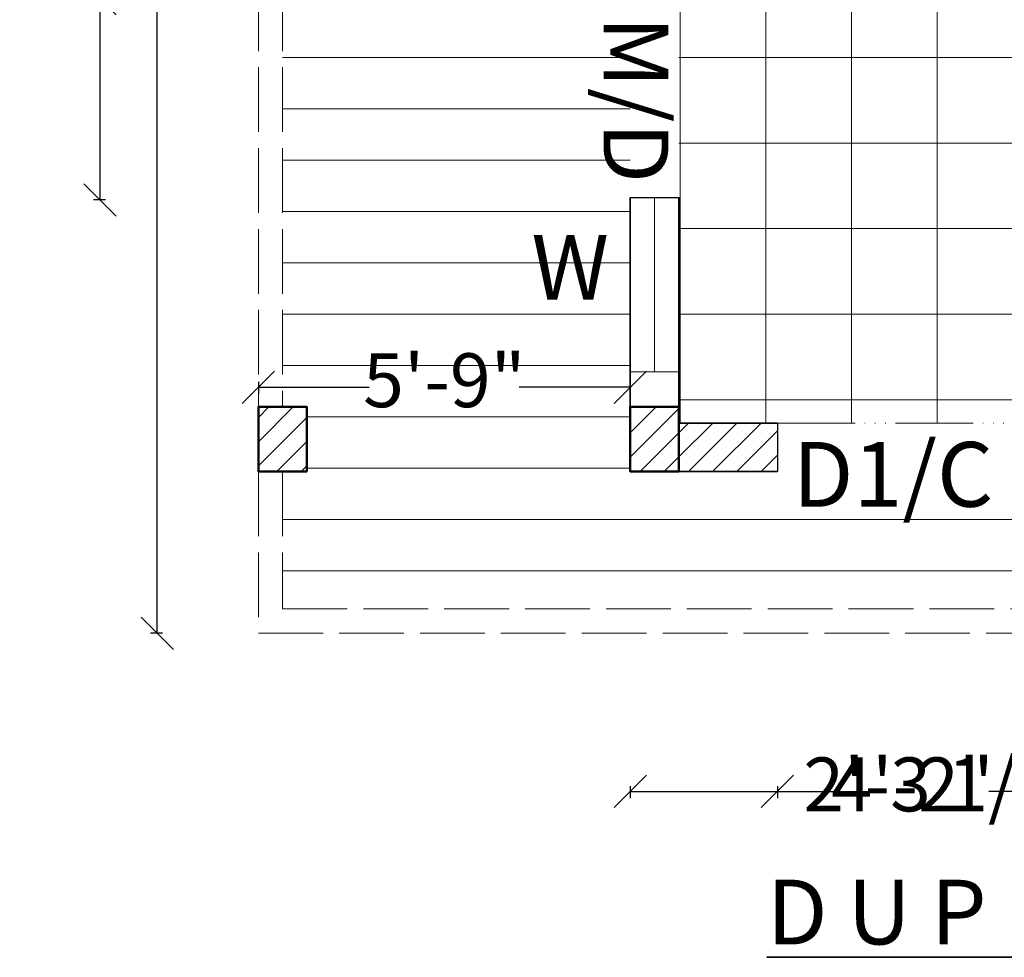
# Model space of a CAD drawing. Units: inches. Extents: x 2036 to 2670, y 319 to 920.
# Tile 1 of 15: x 2036 to 2219, y 405 to 579. Entities that reach past the tile are written whole.
import ezdxf

# ---------------------------------------------------------------- set-up
doc = ezdxf.new("R2010")
doc.units = ezdxf.units.IN
doc.linetypes.add('ACAD_ISO02W100', pattern=[15, 12, -3])
doc.linetypes.add('ACAD_ISO06W100', pattern=[36, 24, -3, 0, -3, 0, -3, 0, -3])
for name, color, linetype, lineweight in [('A-ANNO-DIMS', 2, 'Continuous', 18), ('A-ANNO-TEXT', 7, 'Continuous', 18), ('A-ANNO-TITL', 7, 'Continuous', 35), ('A-COLS', 7, 'Continuous', 50), ('A-DOOR', 3, 'Continuous', 25), ('A-DOOR-OVHD', 3, 'ACAD_ISO06W100', 18), ('A-FLOR-OVHD', 1, 'ACAD_ISO02W100', 13), ('A-FLOR-PATT', 8, 'Continuous', 9), ('A-GLAZ', 4, 'Continuous', 18), ('A-WALL', 7, 'Continuous', 35)]:
    doc.layers.add(name, color=color, linetype=linetype, lineweight=lineweight)
doc.layers.add('A-COLS-PATT', color=240, linetype='Continuous', lineweight=13, true_color=0xed1f24)
doc.layers.add('A-WALL-PATT', color=52, linetype='Continuous', lineweight=13, true_color=0xc8c92d)
doc.styles.get("Standard").update_dxf_attribs({"font": 'arial.ttf'})
doc.dimstyles.new('ISO-25', dxfattribs={"dimtxt": 10, "dimasz": 6, "dimexe": 1.25, "dimexo": 0.625, "dimtad": 0, "dimdec": 1, "dimlunit": 3, "dimtxsty": 'Standard', "dimblk": 'OBLIQUE', "dimcen": 2.5, "dimclrd": 94, "dimclre": 94, "dimclrt": 1, "dimadec": 0, "dimazin": 0, "dimtfac": 1, "dimtdec": 1, "dimtmove": 0, "dimatfit": 3, "dimfxl": 1, "dimfxlon": 1, "dimarcsym": 0})

# ---------------------------------------------------------------- blocks, each defined once
blk = doc.blocks.new('_Oblique')
at = {"color": 0, "linetype": 'ByBlock', "lineweight": -2}
blk.add_line((-0.5, -0.5), (0.5, 0.5), dxfattribs=at)
blk = doc.blocks.new('*D13')
at = {"layer": 'A-ANNO-DIMS', "color": 0, "lineweight": -2, "transparency": 16777216}
for p, q in [((2062.98, 875.68), (2060.73, 875.68)), ((2061.98, 875.68), (2061.98, 687.98)), ((2061.98, 464.68), (2061.98, 652.39)), ((2062.98, 464.68), (2060.73, 464.68))]:
    blk.add_line(p, q, dxfattribs=at)
at = {"layer": 'Defpoints', "color": 0, "transparency": 16777216}
for p in [(2080.74, 875.68), (2061.98, 464.68), (2080.74, 464.68)]:
    blk.add_point(p, dxfattribs=at)
at = {"layer": 'A-ANNO-DIMS', "color": 0, "lineweight": -2, "transparency": 16777216, "xscale": 6, "yscale": 6, "zscale": 6}
for p, rotation in [((2061.98, 875.68), 90), ((2061.98, 464.68), 270)]:
    blk.add_blockref('_Oblique', p, dxfattribs=dict(at, rotation=rotation))
at = {"layer": 'A-ANNO-DIMS', "color": 0, "transparency": 16777216, "insert": (2061.98, 670.18), "char_height": 10, "attachment_point": 5, "rotation": 90}
blk.add_mtext('34\'-3"', dxfattribs=at)
blk = doc.blocks.new('*D15')
at = {"layer": 'A-ANNO-DIMS', "color": 0, "lineweight": -2, "transparency": 16777216}
for p, q in [((2080.74, 511.32), (2080.74, 509.07)), ((2080.74, 510.32), (2101.32, 510.32)), ((2149.74, 510.32), (2129.15, 510.32)), ((2149.74, 511.32), (2149.74, 509.07))]:
    blk.add_line(p, q, dxfattribs=at)
at = {"layer": 'Defpoints', "color": 0, "transparency": 16777216}
for p in [(2080.74, 514.8), (2149.74, 514.8), (2149.74, 510.32)]:
    blk.add_point(p, dxfattribs=at)
at = {"layer": 'A-ANNO-DIMS', "color": 0, "lineweight": -2, "transparency": 16777216, "xscale": 6, "yscale": 6, "zscale": 6, "rotation": 180}
blk.add_blockref('_Oblique', (2080.74, 510.32), dxfattribs=at)
at = {"layer": 'A-ANNO-DIMS', "color": 0, "lineweight": -2, "transparency": 16777216, "xscale": 6, "yscale": 6, "zscale": 6}
blk.add_blockref('_Oblique', (2149.74, 510.32), dxfattribs=at)
at = {"layer": 'A-ANNO-DIMS', "color": 0, "transparency": 16777216, "insert": (2115.24, 510.32), "char_height": 10, "attachment_point": 5}
blk.add_mtext('5\'-9"', dxfattribs=at)
blk = doc.blocks.new('COL-9x12')
blk.add_lwpolyline([(9, 0), (0, 0), (0, 12), (9, 12)], close=True)
blk = doc.blocks.new('*D41')
at = {"layer": 'A-ANNO-DIMS', "color": 94, "lineweight": -2, "transparency": 16777216}
for p, q in [((2149.74, 436.33), (2149.74, 434.08)), ((2149.74, 435.33), (2177.02, 435.33)), ((2177.02, 436.33), (2177.02, 434.08)), ((2177.02, 435.33), (2183.02, 435.33))]:
    blk.add_line(p, q, dxfattribs=at)
at = {"layer": 'Defpoints', "color": 0, "transparency": 16777216}
for p in [(2149.74, 494.68), (2177.02, 494.68), (2177.02, 435.33)]:
    blk.add_point(p, dxfattribs=at)
at = {"layer": 'A-ANNO-DIMS', "color": 94, "lineweight": -2, "transparency": 16777216, "xscale": 6, "yscale": 6, "zscale": 6, "rotation": 180}
blk.add_blockref('_Oblique', (2149.74, 435.33), dxfattribs=at)
at = {"layer": 'A-ANNO-DIMS', "color": 94, "lineweight": -2, "transparency": 16777216, "xscale": 6, "yscale": 6, "zscale": 6}
blk.add_blockref('_Oblique', (2177.02, 435.33), dxfattribs=at)
at = {"layer": 'A-ANNO-DIMS', "color": 1, "transparency": 16777216, "insert": (2208.67, 435.33), "char_height": 10, "attachment_point": 5}
blk.add_mtext('2\'-3 1/2"', dxfattribs=at)
blk = doc.blocks.new('*D42')
at = {"layer": 'A-ANNO-DIMS', "color": 94, "lineweight": -2, "transparency": 16777216}
for p, q in [((2177.02, 436.33), (2177.02, 434.08)), ((2177.02, 435.33), (2187.98, 435.33)), ((2227.17, 435.33), (2216.21, 435.33)), ((2227.17, 436.33), (2227.17, 434.08))]:
    blk.add_line(p, q, dxfattribs=at)
at = {"layer": 'Defpoints', "color": 0, "transparency": 16777216}
for p in [(2177.02, 494.68), (2227.17, 494.68), (2227.17, 435.33)]:
    blk.add_point(p, dxfattribs=at)
at = {"layer": 'A-ANNO-DIMS', "color": 94, "lineweight": -2, "transparency": 16777216, "xscale": 6, "yscale": 6, "zscale": 6, "rotation": 180}
blk.add_blockref('_Oblique', (2177.02, 435.33), dxfattribs=at)
at = {"layer": 'A-ANNO-DIMS', "color": 94, "lineweight": -2, "transparency": 16777216, "xscale": 6, "yscale": 6, "zscale": 6}
blk.add_blockref('_Oblique', (2227.17, 435.33), dxfattribs=at)
at = {"layer": 'A-ANNO-DIMS', "color": 1, "transparency": 16777216, "insert": (2202.09, 435.33), "char_height": 10, "attachment_point": 5}
blk.add_mtext('4\'-2"', dxfattribs=at)
blk = doc.blocks.new('*D54')
at = {"layer": 'A-ANNO-DIMS', "color": 94, "lineweight": -2, "transparency": 16777216}
for p, q in [((2642.09, 545.51), (2642.09, 551.51)), ((2641.09, 545.51), (2643.34, 545.51)), ((2642.09, 513.19), (2642.09, 545.51)), ((2641.09, 513.19), (2643.34, 513.19))]:
    blk.add_line(p, q, dxfattribs=at)
at = {"layer": 'Defpoints', "color": 0, "transparency": 16777216}
for p in [(2158.74, 545.51), (2642.09, 545.51), (2158.74, 513.19)]:
    blk.add_point(p, dxfattribs=at)
at = {"layer": 'A-ANNO-DIMS', "color": 94, "lineweight": -2, "transparency": 16777216, "xscale": 6, "yscale": 6, "zscale": 6}
for p, rotation in [((2642.09, 545.51), 90), ((2642.09, 513.19), 270)]:
    blk.add_blockref('_Oblique', p, dxfattribs=dict(at, rotation=rotation))
at = {"layer": 'A-ANNO-DIMS', "color": 1, "transparency": 16777216, "insert": (2642.09, 577.16), "char_height": 10, "attachment_point": 5, "rotation": 90}
blk.add_mtext('2\'-8 1/2"', dxfattribs=at)
blk = doc.blocks.new('*D55')
at = {"layer": 'A-ANNO-DIMS', "color": 94, "lineweight": -2, "transparency": 16777216}
for p, q in [((2641.09, 582.53), (2643.34, 582.53)), ((2642.09, 582.53), (2642.09, 577.94)), ((2642.09, 545.51), (2642.09, 550.11)), ((2641.09, 545.51), (2643.34, 545.51))]:
    blk.add_line(p, q, dxfattribs=at)
at = {"layer": 'Defpoints', "color": 0, "transparency": 16777216}
for p in [(2158.74, 582.53), (2642.09, 582.53), (2158.74, 545.51)]:
    blk.add_point(p, dxfattribs=at)
at = {"layer": 'A-ANNO-DIMS', "color": 94, "lineweight": -2, "transparency": 16777216, "xscale": 6, "yscale": 6, "zscale": 6}
for p, rotation in [((2642.09, 582.53), 90), ((2642.09, 545.51), 270)]:
    blk.add_blockref('_Oblique', p, dxfattribs=dict(at, rotation=rotation))
at = {"layer": 'A-ANNO-DIMS', "color": 1, "transparency": 16777216, "insert": (2642.09, 564.02), "char_height": 10, "attachment_point": 5, "rotation": 90}
blk.add_mtext('3\'-1"', dxfattribs=at)
blk = doc.blocks.new('*D60')
at = {"layer": 'A-ANNO-DIMS', "color": 94, "lineweight": -2, "transparency": 16777216}
for p, q in [((2051.39, 582.41), (2051.39, 588.41)), ((2052.39, 582.41), (2050.14, 582.41)), ((2051.39, 545.09), (2051.39, 582.41)), ((2052.39, 545.09), (2050.14, 545.09))]:
    blk.add_line(p, q, dxfattribs=at)
at = {"layer": 'Defpoints', "color": 0, "transparency": 16777216}
for p in [(2051.39, 582.41), (2515.24, 582.41), (2515.24, 545.09)]:
    blk.add_point(p, dxfattribs=at)
at = {"layer": 'A-ANNO-DIMS', "color": 94, "lineweight": -2, "transparency": 16777216, "xscale": 6, "yscale": 6, "zscale": 6}
for p, rotation in [((2051.39, 582.41), 90), ((2051.39, 545.09), 270)]:
    blk.add_blockref('_Oblique', p, dxfattribs=dict(at, rotation=rotation))
at = {"layer": 'A-ANNO-DIMS', "color": 1, "transparency": 16777216, "insert": (2051.39, 613.98), "char_height": 10, "attachment_point": 5, "rotation": 90}
blk.add_mtext('3\'-1 1/2"', dxfattribs=at)

msp = doc.modelspace()

# ---------------------------------------------------------------- hatches: boundary and pattern name
at = {"layer": 'A-COLS-PATT'}
h = msp.add_hatch(dxfattribs=at)
h.set_pattern_fill('ANSI31', color=256)
h.paths.add_polyline_path([(2089.74, 875.68), (2080.74, 875.68), (2080.74, 863.68), (2089.74, 863.68)])
h.paths.add_polyline_path([(2089.74, 821.68), (2080.74, 821.68), (2080.74, 809.68), (2089.74, 809.68)])
h.paths.add_polyline_path([(2089.74, 624.2), (2080.74, 624.2), (2080.74, 612.2), (2089.74, 612.2)])
h.paths.add_polyline_path([(2158.74, 506.68), (2149.74, 506.68), (2149.74, 494.68), (2158.74, 494.68)])
h.paths.add_polyline_path([(2158.74, 617.33), (2149.74, 617.33), (2149.74, 605.33), (2158.74, 605.33)])
h.paths.add_polyline_path([(2158.74, 736.18), (2149.74, 736.18), (2149.74, 724.18), (2158.74, 724.18)])
h.paths.add_polyline_path([(2158.74, 852.81), (2149.74, 852.81), (2149.74, 843.81), (2158.74, 843.81)])
h.paths.add_polyline_path([(2161.74, 852.81), (2158.74, 852.81), (2158.74, 843.81), (2161.74, 843.81)])
h.paths.add_polyline_path([(2295.21, 857.66), (2290.74, 857.66), (2290.74, 848.68), (2295.21, 848.68)])
h.paths.add_polyline_path([(2290.74, 857.66), (2283.21, 857.66), (2283.21, 848.66), (2290.74, 848.66)])
h.paths.add_polyline_path([(2443.62, 857.68), (2431.62, 857.68), (2431.62, 848.68), (2443.62, 848.68)])
h.paths.add_polyline_path([(2561.81, 857.68), (2549.81, 857.68), (2549.81, 848.68), (2561.81, 848.68)])
h.paths.add_polyline_path([(2295.24, 737.65), (2290.74, 737.65), (2290.74, 728.68), (2295.24, 728.68)])
h.paths.add_polyline_path([(2309.27, 612.12), (2297.27, 612.12), (2297.27, 603.12), (2309.27, 603.12)])
h.paths.add_polyline_path([(2282.24, 503.68), (2270.24, 503.68), (2270.24, 494.68), (2282.24, 494.68)])
h.paths.add_polyline_path([(2431.74, 746.09), (2427.24, 746.09), (2427.24, 737.09), (2431.74, 737.09)])
h.paths.add_polyline_path([(2439.24, 746.09), (2431.74, 746.09), (2431.74, 737.09), (2439.24, 737.09)])
h.paths.add_polyline_path([(2596.59, 736.59), (2584.59, 736.59), (2584.59, 727.59), (2596.59, 727.59)])
h.paths.add_polyline_path([(2586.39, 623.71), (2574.39, 623.71), (2574.39, 619.18), (2586.39, 619.18)])
h.paths.add_polyline_path([(2586.39, 619.18), (2574.39, 619.18), (2574.39, 614.71), (2586.39, 614.71)])
h.paths.add_polyline_path([(2438.74, 623.68), (2431.24, 623.68), (2431.24, 619.18), (2438.74, 619.18)])
h.paths.add_polyline_path([(2438.74, 619.18), (2431.24, 619.18), (2431.24, 614.68), (2438.74, 614.68)])
h.paths.add_polyline_path([(2431.24, 623.68), (2426.74, 623.68), (2426.74, 614.68), (2431.24, 614.68), (2431.24, 619.18)])
h.paths.add_polyline_path([(2527.24, 503.68), (2515.24, 503.68), (2515.24, 494.68), (2527.24, 494.68)])
h.paths.add_polyline_path([(2590.31, 503.68), (2578.31, 503.68), (2578.31, 494.68), (2590.31, 494.68)])
h = msp.add_hatch(dxfattribs=at)
h.set_pattern_fill('ANSI31', color=256)
h.paths.add_polyline_path([(2089.74, 506.68), (2080.74, 506.68), (2080.74, 494.68), (2089.74, 494.68)])
at = {"layer": 'A-FLOR-PATT'}
h = msp.add_hatch(dxfattribs=at)
h.set_pattern_fill('ANSI31', color=256, scale=5, angle=135)
h.paths.add_polyline_path([(2290.74, 659.68), (2158.74, 659.68), (2158.74, 582.53), (2158.74, 545.51), (2158.74, 503.68), (2426.74, 503.68), (2426.74, 614.68), (2426.74, 623.68), (2426.74, 628.18), (2431.24, 628.18), (2431.24, 623.68), (2438.74, 623.68), (2438.74, 619.18), (2574.39, 619.18), (2574.39, 623.71), (2586.39, 623.71), (2586.39, 619.18), (2603.74, 619.18), (2603.74, 824.68), (2431.74, 824.68), (2431.74, 746.09), (2439.24, 746.09), (2439.24, 737.09), (2431.74, 737.09), (2431.74, 659.68), (2427.24, 659.68), (2427.24, 739.48), (2383.24, 739.48), (2383.24, 804.68), (2339.24, 804.68), (2339.24, 749.08), (2295.24, 749.08), (2295.24, 737.65), (2295.27, 737.65), (2295.27, 728.65), (2295.21, 728.65, -0.586418), (2272.74, 728.68), (2272.74, 824.68), (2270.11, 824.68), (2270.11, 829.18), (2290.74, 829.18), (2290.74, 848.66), (2283.21, 848.66), (2283.21, 857.66), (2289.74, 857.66), (2289.74, 874.68), (2158.74, 874.68), (2158.74, 852.81), (2161.74, 852.81), (2161.74, 843.81), (2158.74, 843.81), (2158.74, 829.18), (2224.74, 829.18), (2224.74, 800.68), (2182.74, 800.68), (2182.74, 733.41), (2158.74, 733.41), (2158.74, 728.68), (2235.24, 728.68), (2235.24, 714.81), (2230.74, 714.81), (2230.74, 724.18), (2158.74, 724.18), (2158.74, 664.18), (2230.74, 664.18), (2230.74, 678.81), (2235.24, 678.81), (2235.24, 664.18), (2290.74, 664.18)])
h.paths.add_polyline_path([(2309.27, 612.12), (2309.27, 603.12), (2297.27, 603.12), (2297.27, 612.12)], flags=16)
h.paths.add_polyline_path([(2280.12, 639.11), (2280.26, 638.18, -0.414214), (2279.26, 637.18), (2278.76, 637.18), (2279.26, 633.18), (2277.76, 633.18), (2277.26, 637.18), (2269.76, 637.18), (2262.26, 637.18), (2261.76, 633.18), (2260.26, 633.18), (2260.76, 637.18), (2260.26, 637.18, -0.414214), (2259.26, 638.18), (2259.41, 639.11, -0.541164), (2257.76, 641.18), (2260.76, 652.18), (2261.45, 652.18), (2261.53, 652.68), (2262.76, 652.68), (2262.25, 655.24, 0.001913), (2261.76, 655.18), (2259.76, 658.18, -0.15), (2279.76, 658.18), (2277.76, 655.18, 0.001913), (2277.27, 655.24), (2276.76, 652.68), (2278, 652.68), (2278.07, 652.18), (2278.76, 652.18), (2281.76, 641.18, -0.541163)], flags=16)
h.paths.add_polyline_path([(2245.98, 639.11), (2246.13, 638.18, -0.414214), (2245.13, 637.18), (2244.63, 637.18), (2245.13, 633.18), (2243.63, 633.18), (2243.13, 637.18), (2235.63, 637.18), (2228.13, 637.18), (2227.63, 633.18), (2226.13, 633.18), (2226.63, 637.18), (2226.13, 637.18, -0.414214), (2225.13, 638.18), (2225.27, 639.11, -0.541164), (2223.63, 641.18), (2226.63, 652.18), (2227.32, 652.18), (2227.39, 652.68), (2228.63, 652.68), (2228.12, 655.24, 0.001913), (2227.63, 655.18), (2225.63, 658.18, -0.15), (2245.63, 658.18), (2243.63, 655.18, 0.001913), (2243.14, 655.24), (2242.63, 652.68), (2243.86, 652.68), (2243.94, 652.18), (2244.63, 652.18), (2247.63, 641.18, -0.541163)], flags=16)
h.paths.add_polyline_path([(2351.59, 515.15, -0.151948), (2279.59, 515.15), (2279.59, 537.68), (2273.59, 537.68), (2273.59, 511.68, 0.190476), (2357.59, 511.68), (2357.59, 537.68), (2351.59, 537.68)])
h.paths.add_polyline_path([(2327.59, 536.13), (2327.59, 517.07), (2303.59, 517.07), (2303.59, 536.13)], flags=16)
h.paths.add_polyline_path([(2213.4, 639.11), (2213.55, 638.18, -0.414214), (2212.55, 637.18), (2212.05, 637.18), (2212.55, 633.18), (2211.05, 633.18), (2210.55, 637.18), (2203.05, 637.18), (2195.55, 637.18), (2195.05, 633.18), (2193.55, 633.18), (2194.05, 637.18), (2193.55, 637.18, -0.414214), (2192.55, 638.18), (2192.69, 639.11, -0.541164), (2191.05, 641.18), (2194.05, 652.18), (2194.73, 652.18), (2194.81, 652.68), (2196.05, 652.68), (2195.53, 655.24, 0.001913), (2195.05, 655.18), (2193.05, 658.18, -0.15), (2213.05, 658.18), (2211.05, 655.18, 0.001913), (2210.56, 655.24), (2210.05, 652.68), (2211.28, 652.68), (2211.36, 652.18), (2212.05, 652.18), (2215.05, 641.18, -0.541163)], flags=16)
h.paths.add_polyline_path([(2368.58, 538.02), (2370.52, 538.02), (2371.17, 532.84), (2380.89, 532.84), (2390.6, 532.84), (2391.25, 538.02), (2393.2, 538.02), (2392.55, 532.84), (2380.89, 532.84), (2368.58, 532.84, 0.414214), (2367.28, 531.54), (2367.47, 530.34, -0.483352), (2369.23, 527.65), (2371.82, 513.4), (2370.12, 513.4), (2370.22, 512.75), (2391.56, 512.75), (2391.66, 513.4), (2389.96, 513.4), (2392.55, 527.65, -1.387427), (2396.43, 527.65), (2392.55, 513.4), (2391.66, 513.4), (2391.56, 512.75), (2389.31, 512.75), (2390, 509.37, 0.003796), (2391.25, 509.51), (2393.84, 505.63, -0.15), (2367.93, 505.63), (2370.52, 509.51, 0.003901), (2371.81, 509.36), (2372.47, 512.75), (2370.22, 512.75), (2370.12, 513.4), (2369.23, 513.4), (2365.34, 527.65, -0.541163), (2367.47, 530.34), (2367.28, 531.54, -0.414214), (2368.58, 532.84), (2369.23, 532.84)])
h.paths.add_polyline_path([(2266.74, 538.02), (2266.09, 532.84), (2254.43, 532.84), (2242.12, 532.84, 0.414214), (2240.83, 531.54), (2241.01, 530.34, -0.483352), (2242.77, 527.65), (2245.36, 513.4), (2243.66, 513.4), (2243.76, 512.75), (2265.1, 512.75), (2265.2, 513.4), (2263.5, 513.4), (2266.09, 527.65, -1.387427), (2269.98, 527.65), (2266.09, 513.4), (2265.2, 513.4), (2265.1, 512.75), (2262.85, 512.75), (2263.54, 509.37, 0.003796), (2264.79, 509.51), (2267.39, 505.63, -0.15), (2241.47, 505.63), (2244.07, 509.51, 0.003901), (2245.36, 509.36), (2246.01, 512.75), (2243.76, 512.75), (2243.66, 513.4), (2242.77, 513.4), (2238.88, 527.65, -0.541163), (2241.01, 530.34), (2240.83, 531.54, -0.414214), (2242.12, 532.84), (2242.77, 532.84), (2242.12, 538.02), (2244.07, 538.02), (2244.71, 532.84), (2254.43, 532.84), (2264.15, 532.84), (2264.79, 538.02)])
h.paths.add_polyline_path([(2185.24, 620.36), (2185.24, 618.86), (2181.24, 618.36), (2181.24, 610.86), (2181.24, 603.36), (2185.24, 602.86), (2185.24, 601.36), (2181.24, 601.86), (2181.24, 601.36, -0.414214), (2180.24, 600.36), (2179.31, 600.5, -0.541164), (2177.24, 598.86), (2166.24, 601.86), (2166.24, 602.54), (2165.74, 602.62), (2165.74, 603.86), (2163.18, 603.34, 0.001913), (2163.24, 602.86), (2160.24, 600.86, -0.15), (2160.24, 620.86), (2163.24, 618.86, 0.001913), (2163.18, 618.37), (2165.74, 617.86), (2165.74, 619.09), (2166.24, 619.17), (2166.24, 619.86), (2177.24, 622.86, -0.541163), (2179.31, 621.21), (2180.24, 621.36, -0.414214), (2181.24, 620.36), (2181.24, 619.86)])
h.paths.add_polyline_path([(2470.92, 676.01), (2470.92, 806.13), (2568.52, 806.13), (2568.52, 676.01)], flags=16)
h.paths.add_polyline_path([(2177.74, 677.49), (2161.9, 677.49), (2161.9, 705.85), (2177.74, 705.85)], flags=16)
h.paths.add_polyline_path([(2176.74, 678.49), (2162.9, 678.49), (2162.9, 704.85), (2176.74, 704.85)], flags=0)
h.paths.add_polyline_path([(2175.01, 686.48), (2172.93, 686.48), (2172.93, 690.63), (2170.86, 690.63), (2170.86, 686.48), (2164.63, 686.48), (2164.63, 688.56), (2166.71, 688.56), (2168.78, 688.56), (2168.78, 690.63), (2164.63, 690.63), (2164.63, 696.85), (2166.71, 696.85), (2166.71, 692.71), (2168.78, 692.71), (2168.78, 696.85), (2175.01, 696.85), (2175.01, 694.78), (2170.86, 694.78), (2170.86, 692.71), (2175.01, 692.71)], flags=0)
h.paths.add_polyline_path([(2543.79, 782.71), (2483.94, 782.71), (2483.94, 804.18), (2517.77, 804.18), (2517.77, 782.71), (2521.67, 782.71), (2521.67, 804.18), (2555.5, 804.18), (2555.5, 779.45), (2547.05, 779.45), (2568.52, 757.98), (2543.79, 757.98)], flags=0)
h.paths.add_polyline_path([(2584.59, 727.59), (2584.59, 736.59), (2596.59, 736.59), (2596.59, 727.59)], flags=16)
h.paths.add_polyline_path([(2520.45, 647.03), (2553.79, 647.03), (2553.79, 658.23), (2520.45, 658.23)], flags=24)
h.paths.add_polyline_path([(2299.53, 573.74), (2331.71, 573.74), (2331.71, 584.94), (2299.53, 584.94)], flags=24)
h.paths.add_polyline_path([(2191.59, 685.19), (2212.12, 685.19), (2212.12, 696.38), (2191.59, 696.38)], flags=24)
h.paths.add_polyline_path([(2353.9, 649.86), (2379.08, 649.86), (2379.08, 661.06), (2353.9, 661.06)], flags=24)
h.paths.add_polyline_path([(2214.61, 763.31), (2237.46, 763.31), (2237.46, 779.56), (2214.61, 779.56)], flags=24)
h.paths.add_polyline_path([(2225.09, 819.31), (2269.29, 819.31), (2269.29, 844.04), (2225.09, 844.04)], flags=24)
h.paths.add_polyline_path([(2204.06, 845.04), (2226.92, 845.04), (2226.92, 856.24), (2204.06, 856.24)], flags=24)
h = msp.add_hatch(dxfattribs=at)
h.set_pattern_fill('ANSI31', color=256, scale=5, angle=45)
h.paths.add_polyline_path([(2290.74, 659.68), (2158.74, 659.68), (2158.74, 582.53), (2158.74, 545.51), (2158.74, 503.68), (2426.74, 503.68), (2426.74, 614.68), (2426.74, 623.68), (2426.74, 628.18), (2431.24, 628.18), (2431.24, 623.68), (2438.74, 623.68), (2438.74, 619.18), (2574.39, 619.18), (2574.39, 623.71), (2586.39, 623.71), (2586.39, 619.18), (2603.74, 619.18), (2603.74, 824.68), (2431.74, 824.68), (2431.74, 746.09), (2439.24, 746.09), (2439.24, 737.09), (2431.74, 737.09), (2431.74, 659.68), (2427.24, 659.68), (2427.24, 739.48), (2383.24, 739.48), (2383.24, 804.68), (2339.24, 804.68), (2339.24, 749.08), (2295.24, 749.08), (2295.24, 737.65), (2295.27, 737.65), (2295.27, 728.65), (2295.21, 728.65, -0.586418), (2272.74, 728.68), (2272.74, 824.68), (2270.11, 824.68), (2270.11, 829.18), (2290.74, 829.18), (2290.74, 848.66), (2283.21, 848.66), (2283.21, 857.66), (2289.74, 857.66), (2289.74, 874.68), (2158.74, 874.68), (2158.74, 852.81), (2161.74, 852.81), (2161.74, 843.81), (2158.74, 843.81), (2158.74, 829.18), (2224.74, 829.18), (2224.74, 800.68), (2182.74, 800.68), (2182.74, 733.41), (2158.74, 733.41), (2158.74, 728.68), (2235.24, 728.68), (2235.24, 714.81), (2230.74, 714.81), (2230.74, 724.18), (2158.74, 724.18), (2158.74, 664.18), (2230.74, 664.18), (2230.74, 678.81), (2235.24, 678.81), (2235.24, 664.18), (2290.74, 664.18)])
h.paths.add_polyline_path([(2309.27, 612.12), (2309.27, 603.12), (2297.27, 603.12), (2297.27, 612.12)], flags=16)
h.paths.add_polyline_path([(2280.12, 639.11), (2280.26, 638.18, -0.414214), (2279.26, 637.18), (2278.76, 637.18), (2279.26, 633.18), (2277.76, 633.18), (2277.26, 637.18), (2269.76, 637.18), (2262.26, 637.18), (2261.76, 633.18), (2260.26, 633.18), (2260.76, 637.18), (2260.26, 637.18, -0.414214), (2259.26, 638.18), (2259.41, 639.11, -0.541164), (2257.76, 641.18), (2260.76, 652.18), (2261.45, 652.18), (2261.53, 652.68), (2262.76, 652.68), (2262.25, 655.24, 0.001913), (2261.76, 655.18), (2259.76, 658.18, -0.15), (2279.76, 658.18), (2277.76, 655.18, 0.001913), (2277.27, 655.24), (2276.76, 652.68), (2278, 652.68), (2278.07, 652.18), (2278.76, 652.18), (2281.76, 641.18, -0.541163)], flags=16)
h.paths.add_polyline_path([(2245.98, 639.11), (2246.13, 638.18, -0.414214), (2245.13, 637.18), (2244.63, 637.18), (2245.13, 633.18), (2243.63, 633.18), (2243.13, 637.18), (2235.63, 637.18), (2228.13, 637.18), (2227.63, 633.18), (2226.13, 633.18), (2226.63, 637.18), (2226.13, 637.18, -0.414214), (2225.13, 638.18), (2225.27, 639.11, -0.541164), (2223.63, 641.18), (2226.63, 652.18), (2227.32, 652.18), (2227.39, 652.68), (2228.63, 652.68), (2228.12, 655.24, 0.001913), (2227.63, 655.18), (2225.63, 658.18, -0.15), (2245.63, 658.18), (2243.63, 655.18, 0.001913), (2243.14, 655.24), (2242.63, 652.68), (2243.86, 652.68), (2243.94, 652.18), (2244.63, 652.18), (2247.63, 641.18, -0.541163)], flags=16)
h.paths.add_polyline_path([(2351.59, 537.68), (2351.59, 515.15, -0.151948), (2279.59, 515.15), (2279.59, 537.68), (2273.59, 537.68), (2273.59, 511.68, 0.190476), (2357.59, 511.68), (2357.59, 537.68)])
h.paths.add_polyline_path([(2368.58, 538.02), (2370.52, 538.02), (2371.17, 532.84), (2380.89, 532.84), (2390.6, 532.84), (2391.25, 538.02), (2393.2, 538.02), (2392.55, 532.84), (2380.89, 532.84), (2368.58, 532.84, 0.414214), (2367.28, 531.54), (2367.47, 530.34, -0.483352), (2369.23, 527.65), (2371.82, 513.4), (2370.12, 513.4), (2370.22, 512.75), (2391.56, 512.75), (2391.66, 513.4), (2389.96, 513.4), (2392.55, 527.65, -1.387427), (2396.43, 527.65), (2392.55, 513.4), (2391.66, 513.4), (2391.56, 512.75), (2389.31, 512.75), (2390, 509.37, 0.003796), (2391.25, 509.51), (2393.84, 505.63, -0.15), (2367.93, 505.63), (2370.52, 509.51, 0.003901), (2371.81, 509.36), (2372.47, 512.75), (2370.22, 512.75), (2370.12, 513.4), (2369.23, 513.4), (2365.34, 527.65, -0.541163), (2367.47, 530.34), (2367.28, 531.54, -0.414214), (2368.58, 532.84), (2369.23, 532.84)])
h.paths.add_polyline_path([(2327.59, 536.13), (2327.59, 517.07), (2303.59, 517.07), (2303.59, 536.13)], flags=16)
h.paths.add_polyline_path([(2470.92, 676.01), (2470.92, 806.13), (2568.52, 806.13), (2568.52, 676.01)], flags=16)
h.paths.add_polyline_path([(2266.74, 538.02), (2266.09, 532.84), (2254.43, 532.84), (2242.12, 532.84, 0.414214), (2240.83, 531.54), (2241.01, 530.34, -0.483352), (2242.77, 527.65), (2245.36, 513.4), (2243.66, 513.4), (2243.76, 512.75), (2265.1, 512.75), (2265.2, 513.4), (2263.5, 513.4), (2266.09, 527.65, -1.387427), (2269.98, 527.65), (2266.09, 513.4), (2265.2, 513.4), (2265.1, 512.75), (2262.85, 512.75), (2263.54, 509.37, 0.003796), (2264.79, 509.51), (2267.39, 505.63, -0.15), (2241.47, 505.63), (2244.07, 509.51, 0.003901), (2245.36, 509.36), (2246.01, 512.75), (2243.76, 512.75), (2243.66, 513.4), (2242.77, 513.4), (2238.88, 527.65, -0.541163), (2241.01, 530.34), (2240.83, 531.54, -0.414214), (2242.12, 532.84), (2242.77, 532.84), (2242.12, 538.02), (2244.07, 538.02), (2244.71, 532.84), (2254.43, 532.84), (2264.15, 532.84), (2264.79, 538.02)])
h.paths.add_polyline_path([(2213.4, 639.11), (2213.55, 638.18, -0.414214), (2212.55, 637.18), (2212.05, 637.18), (2212.55, 633.18), (2211.05, 633.18), (2210.55, 637.18), (2203.05, 637.18), (2195.55, 637.18), (2195.05, 633.18), (2193.55, 633.18), (2194.05, 637.18), (2193.55, 637.18, -0.414214), (2192.55, 638.18), (2192.69, 639.11, -0.541164), (2191.05, 641.18), (2194.05, 652.18), (2194.73, 652.18), (2194.81, 652.68), (2196.05, 652.68), (2195.53, 655.24, 0.001913), (2195.05, 655.18), (2193.05, 658.18, -0.15), (2213.05, 658.18), (2211.05, 655.18, 0.001913), (2210.56, 655.24), (2210.05, 652.68), (2211.28, 652.68), (2211.36, 652.18), (2212.05, 652.18), (2215.05, 641.18, -0.541163)], flags=16)
h.paths.add_polyline_path([(2185.24, 620.36), (2185.24, 618.86), (2181.24, 618.36), (2181.24, 610.86), (2181.24, 603.36), (2185.24, 602.86), (2185.24, 601.36), (2181.24, 601.86), (2181.24, 601.36, -0.414214), (2180.24, 600.36), (2179.31, 600.5, -0.541164), (2177.24, 598.86), (2166.24, 601.86), (2166.24, 602.54), (2165.74, 602.62), (2165.74, 603.86), (2163.18, 603.34, 0.001913), (2163.24, 602.86), (2160.24, 600.86, -0.15), (2160.24, 620.86), (2163.24, 618.86, 0.001913), (2163.18, 618.37), (2165.74, 617.86), (2165.74, 619.09), (2166.24, 619.17), (2166.24, 619.86), (2177.24, 622.86, -0.541163), (2179.31, 621.21), (2180.24, 621.36, -0.414214), (2181.24, 620.36), (2181.24, 619.86)])
h.paths.add_polyline_path([(2177.74, 677.49), (2161.9, 677.49), (2161.9, 705.85), (2177.74, 705.85)], flags=16)
h.paths.add_polyline_path([(2176.74, 678.49), (2162.9, 678.49), (2162.9, 704.85), (2176.74, 704.85)], flags=0)
h.paths.add_polyline_path([(2175.01, 686.48), (2172.93, 686.48), (2172.93, 690.63), (2170.86, 690.63), (2170.86, 686.48), (2164.63, 686.48), (2164.63, 688.56), (2166.71, 688.56), (2168.78, 688.56), (2168.78, 690.63), (2164.63, 690.63), (2164.63, 696.85), (2166.71, 696.85), (2166.71, 692.71), (2168.78, 692.71), (2168.78, 696.85), (2175.01, 696.85), (2175.01, 694.78), (2170.86, 694.78), (2170.86, 692.71), (2175.01, 692.71)], flags=0)
h.paths.add_polyline_path([(2543.79, 782.71), (2483.94, 782.71), (2483.94, 804.18), (2517.77, 804.18), (2517.77, 782.71), (2521.67, 782.71), (2521.67, 804.18), (2555.5, 804.18), (2555.5, 779.45), (2547.05, 779.45), (2568.52, 757.98), (2543.79, 757.98)], flags=0)
h.paths.add_polyline_path([(2584.59, 727.59), (2584.59, 736.59), (2596.59, 736.59), (2596.59, 727.59)], flags=16)
h.paths.add_polyline_path([(2520.45, 647.03), (2553.79, 647.03), (2553.79, 658.23), (2520.45, 658.23)], flags=24)
h.paths.add_polyline_path([(2299.53, 573.74), (2331.71, 573.74), (2331.71, 584.94), (2299.53, 584.94)], flags=24)
h.paths.add_polyline_path([(2191.59, 685.19), (2212.12, 685.19), (2212.12, 696.38), (2191.59, 696.38)], flags=24)
h.paths.add_polyline_path([(2353.9, 649.86), (2379.08, 649.86), (2379.08, 661.06), (2353.9, 661.06)], flags=24)
h.paths.add_polyline_path([(2214.61, 763.31), (2237.46, 763.31), (2237.46, 779.56), (2214.61, 779.56)], flags=24)
h.paths.add_polyline_path([(2225.09, 819.31), (2269.29, 819.31), (2269.29, 844.04), (2225.09, 844.04)], flags=24)
h.paths.add_polyline_path([(2204.06, 845.04), (2226.92, 845.04), (2226.92, 856.24), (2204.06, 856.24)], flags=24)
h = msp.add_hatch(dxfattribs=at)
h.set_pattern_fill('ANSI31', color=256, scale=3, angle=135)
h.paths.add_polyline_path([(2149.74, 582.53), (2149.74, 707.68), (2120.74, 707.68), (2120.74, 599.68, -1), (2118.74, 599.68), (2085.24, 599.68), (2085.24, 506.68), (2089.74, 506.68), (2089.74, 494.68), (2085.24, 494.68), (2085.24, 469.18), (2608.24, 469.18), (2608.24, 494.68), (2149.74, 494.68), (2149.74, 506.68), (2149.74, 545.51)])
h.paths.add_polyline_path([(2143.58, 686.71), (2149.03, 686.71), (2149.03, 692.89), (2143.58, 692.89)], flags=24)
h.paths.add_polyline_path([(2125.99, 700.31), (2133.31, 700.31), (2133.31, 706.49), (2125.99, 706.49)], flags=24)
at = {"layer": 'A-WALL-PATT'}
h = msp.add_hatch(dxfattribs=at)
h.set_pattern_fill('ANSI31', color=256)
h.paths.add_polyline_path([(2089.74, 863.68), (2080.74, 863.68), (2080.74, 821.68), (2089.74, 821.68)])
h.paths.add_polyline_path([(2089.74, 809.68), (2080.74, 809.68), (2080.74, 624.2), (2089.74, 624.2), (2089.74, 707.68), (2089.74, 767.68)])
h.paths.add_polyline_path([(2149.74, 818.68), (2089.74, 818.68), (2089.74, 809.68), (2149.74, 809.68)])
h.paths.add_polyline_path([(2158.74, 875.68), (2089.74, 875.68), (2089.74, 866.68), (2149.74, 866.68), (2149.74, 852.81), (2158.74, 852.81)])
h.paths.add_polyline_path([(2158.74, 843.81), (2149.74, 843.81), (2149.74, 736.18), (2158.74, 736.18), (2158.74, 824.68)])
h.paths.add_polyline_path([(2181.31, 829.18), (2158.74, 829.18), (2158.74, 824.68), (2181.31, 824.68)])
h.paths.add_polyline_path([(2224.74, 829.18), (2212.72, 829.18), (2212.72, 824.68), (2224.74, 824.68)])
h.paths.add_polyline_path([(2177.02, 503.68), (2158.74, 503.68), (2158.74, 494.68), (2177.02, 494.68)])
h.paths.add_polyline_path([(2158.74, 664.18), (2158.74, 680.02), (2149.74, 680.02), (2149.74, 617.33), (2158.74, 617.33)])
h.paths.add_polyline_path([(2158.74, 724.18), (2149.74, 724.18), (2149.74, 704.02), (2158.74, 704.02)])
h.paths.add_polyline_path([(2235.24, 728.68), (2158.74, 728.68), (2158.74, 724.18), (2230.74, 724.18), (2230.74, 714.81), (2235.24, 714.81)])
h.paths.add_polyline_path([(2290.74, 664.18), (2235.24, 664.18), (2235.24, 678.81), (2230.74, 678.81), (2230.74, 664.18), (2158.74, 664.18), (2158.74, 659.68), (2290.74, 659.68)])
h.paths.add_polyline_path([(2270.24, 503.68), (2227.17, 503.68), (2227.17, 494.68), (2270.24, 494.68)])
h.paths.add_polyline_path([(2515.24, 503.68), (2380.89, 503.68), (2380.89, 494.68), (2515.24, 494.68)])
h.paths.add_polyline_path([(2292.21, 503.68), (2282.24, 503.68), (2282.24, 494.68), (2292.21, 494.68)])
h.paths.add_polyline_path([(2578.31, 503.68), (2527.24, 503.68), (2527.24, 494.68), (2578.31, 494.68)])
h.paths.add_polyline_path([(2603.74, 503.68), (2590.31, 503.68), (2590.31, 494.68), (2603.74, 494.68)])
h.paths.add_polyline_path([(2612.74, 503.68), (2603.74, 503.68), (2603.74, 494.68), (2612.74, 494.68)])
h.paths.add_polyline_path([(2549.81, 857.68), (2443.62, 857.68), (2443.62, 848.68), (2549.81, 848.68)])
h.paths.add_polyline_path([(2295.24, 848.66), (2290.74, 848.66), (2290.74, 829.18), (2270.11, 829.18), (2270.11, 824.68), (2290.74, 824.68), (2290.74, 737.65), (2295.24, 737.65)])
h.paths.add_polyline_path([(2431.74, 737.09), (2427.24, 737.09), (2427.24, 659.68), (2431.74, 659.68)])
h.paths.add_polyline_path([(2431.74, 848.68), (2427.24, 848.68), (2427.24, 746.09), (2431.74, 746.09)])
h.paths.add_polyline_path([(2574.39, 619.18), (2495.46, 619.18), (2495.46, 614.68), (2574.39, 614.68)])
h.paths.add_polyline_path([(2461.84, 619.18), (2438.74, 619.18), (2438.74, 614.68), (2461.84, 614.68)])
h.paths.add_polyline_path([(2603.74, 619.18), (2586.39, 619.18), (2586.39, 614.68), (2603.74, 614.68)], flags=17)

# ---------------------------------------------------------------- linework, layer by layer
at = {"layer": 'A-COLS'}
msp.add_lwpolyline([(2089.74, 494.68), (2080.74, 494.68), (2080.74, 506.68), (2089.74, 506.68)], close=True, dxfattribs=at)
at = {"layer": 'A-DOOR'}
for p, q in [((2149.74, 545.51), (2158.74, 545.51)), ((2177.02, 503.68), (2177.02, 494.68))]:
    msp.add_line(p, q, dxfattribs=at)
at = {"layer": 'A-DOOR-OVHD', "ltscale": 0.6}
msp.add_line((2177.02, 503.68), (2227.17, 503.68), dxfattribs=at)
at = {"layer": 'A-FLOR-OVHD'}
for p, q in [((2080.74, 599.68), (2080.74, 464.68)), ((2085.24, 599.68), (2085.24, 506.68)), ((2085.24, 494.68), (2085.24, 469.18)), ((2085.24, 469.18), (2608.24, 469.18)), ((2080.74, 464.68), (2612.74, 464.68))]:
    msp.add_line(p, q, dxfattribs=at)
at = {"layer": 'A-GLAZ'}
for p, q in [((2154.24, 513.19), (2154.24, 545.51)), ((2149.74, 513.19), (2158.74, 513.19))]:
    msp.add_line(p, q, dxfattribs=at)
at = {"layer": 'A-WALL'}
for p, q in [((2149.74, 545.51), (2149.74, 494.68)), ((2158.74, 545.51), (2158.74, 503.68)), ((2158.74, 503.68), (2177.02, 503.68)), ((2149.74, 494.68), (2177.02, 494.68))]:
    msp.add_line(p, q, dxfattribs=at)

# ---------------------------------------------------------------- block references
at = {"layer": 'A-COLS'}
msp.add_blockref('COL-9x12', (2149.74, 494.68), dxfattribs=at)

# ---------------------------------------------------------------- texts
at = {"layer": 'A-ANNO-TEXT', "insert": (2156.79, 579.16), "char_height": 12, "attachment_point": 1, "rotation": 270}
msp.add_mtext_dynamic_manual_height_columns('M/D', width=22.4417, gutter_width=12.5, heights=[0], dxfattribs=at)
at = {"layer": 'A-ANNO-TEXT', "char_height": 12, "attachment_point": 1}
for s, width, insert in [('W', 27.6972, (2131.4, 538.54)), ('D1/C', 40.6946, (2179.86, 500.15))]:
    msp.add_mtext_dynamic_manual_height_columns(s, width=width, gutter_width=12.5, heights=[0], dxfattribs=dict(at, insert=insert))
at = {"layer": 'A-ANNO-TITL', "insert": (2175.07, 418.94), "char_height": 12, "attachment_point": 1}
msp.add_mtext_dynamic_manual_height_columns('{\\LD U P L E  X   S E C O N D   F L O O R}', width=344.7128, gutter_width=12.5, heights=[0], dxfattribs=at)

# ---------------------------------------------------------------- dimensions: what is measured, and where the dimension line sits
at = {"layer": 'A-ANNO-DIMS'}
for base, p1, p2, override, picture, middle in [((2061.98, 464.68), (2080.74, 875.68), (2080.74, 464.68), {"dimclrd": 0, "dimclre": 0, "dimclrt": 0}, '*D13', (2061.98, 670.18)), ((2051.39, 582.41), (2515.24, 545.09), (2515.24, 582.41), {"dimdec": 1, "dimlfac": 1, "dimrnd": 0, "dimzin": 1, "dimdsep": 46, "dimlunit": 4, "dimfrac": 2}, '*D60', (2051.39, 613.98)), ((2642.09, 545.51), (2158.74, 513.19), (2158.74, 545.51), {"dimdec": 1, "dimlfac": 1, "dimrnd": 0, "dimzin": 1, "dimdsep": 46, "dimlunit": 4, "dimfrac": 2}, '*D54', (2642.09, 577.16)), ((2642.09, 582.53), (2158.74, 545.51), (2158.74, 582.53), {"dimdec": 1, "dimlfac": 1, "dimrnd": 0, "dimzin": 1, "dimdsep": 46, "dimlunit": 4, "dimfrac": 2}, '*D55', (2642.09, 564.02))]:
    dim = msp.add_linear_dim(base=base, p1=p1, p2=p2, angle=90, dimstyle='ISO-25', override=override, dxfattribs=at)
    dim.commit()
    dim.dimension.update_dxf_attribs({"geometry": picture, "text_midpoint": middle})
for base, p1, p2, override, picture, middle in [((2149.74, 510.32), (2080.74, 514.8), (2149.74, 514.8), {"dimclrd": 0, "dimclre": 0, "dimclrt": 0}, '*D15', (2115.24, 510.32)), ((2177.02, 435.33), (2149.74, 494.68), (2177.02, 494.68), {"dimdec": 1, "dimlfac": 1, "dimrnd": 0, "dimzin": 1, "dimdsep": 46, "dimlunit": 4, "dimfrac": 2}, '*D41', (2208.67, 435.33)), ((2227.168, 435.3346), (2177.0218, 494.6846), (2227.168, 494.6846), {"dimdec": 1, "dimlfac": 1, "dimrnd": 0, "dimzin": 1, "dimdsep": 46, "dimlunit": 4, "dimfrac": 2}, '*D42', (2202.0949, 435.3346))]:
    dim = msp.add_linear_dim(base=base, p1=p1, p2=p2, dimstyle='ISO-25', override=override, dxfattribs=at)
    dim.commit()
    dim.dimension.update_dxf_attribs({"geometry": picture, "text_midpoint": middle})

doc.saveas('drawing.dxf')
